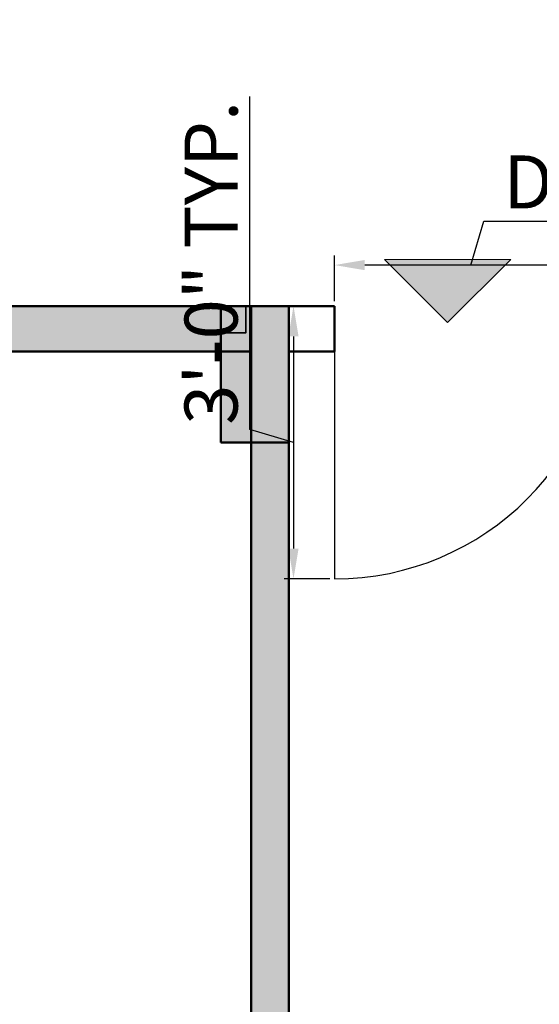
# Model space of a CAD drawing. Units: inches. Extents: x -7 to 1228, y -146 to 1091.
# Tile 14 of 88: x 200 to 269, y 401 to 531. Entities that reach past the tile are written whole.
import ezdxf

# ---------------------------------------------------------------- set-up
doc = ezdxf.new("R2010")
doc.units = ezdxf.units.IN
for name, color, linetype, lineweight in [('A-ANNO-DIMS', 2, 'Continuous', 18), ('A-ANNO-SYMB', 30, 'Continuous', 18), ('A-COLS', 6, 'Continuous', 35), ('A-DOOR', 4, 'Continuous', 25), ('A-WALL', 7, 'Continuous', 50), ('A-WALL-PATT', 251, 'Continuous', 13)]:
    doc.layers.add(name, color=color, linetype=linetype, lineweight=lineweight)
doc.styles.get("Standard").update_dxf_attribs({"font": 'arial.ttf'})
doc.dimstyles.new('ISO-25', dxfattribs={"dimtxt": 7, "dimasz": 4, "dimexe": 1.25, "dimexo": 0.625, "dimtad": 1, "dimdec": 1, "dimlunit": 3, "dimtxsty": 'Standard', "dimcen": 2.5, "dimadec": 0, "dimazin": 0, "dimtfac": 1, "dimtdec": 1, "dimtmove": 1, "dimatfit": 3, "dimfxl": 1, "dimarcsym": 0})

# ---------------------------------------------------------------- blocks, each defined once
blk = doc.blocks.new('DOOR-900')
blk.add_line((36, 0), (36, 36))
blk.add_arc((36, 0), 36, 90, 180)
blk = doc.blocks.new('*D44')
at = {"layer": 'A-ANNO-DIMS', "color": 0, "lineweight": -2, "transparency": 16777216}
for p, q in [((260, 498.4), (261.74, 504.21)), ((261.74, 504.21), (352.58, 504.21)), ((242, 493.62), (242, 499.65)), ((278, 493.62), (278, 499.65)), ((274, 498.4), (246, 498.4))]:
    blk.add_line(p, q, dxfattribs=at)
at = {"layer": 'A-ANNO-DIMS', "color": 0, "transparency": 16777216}
for points in [[(246, 499.07), (246, 497.73), (242, 498.4)], [(274, 499.07), (274, 497.73), (278, 498.4)]]:
    blk.add_solid(points, dxfattribs=at)
at = {"layer": 'Defpoints', "color": 0, "transparency": 16777216}
for p in [(242, 498.4), (242, 493), (278, 493)]:
    blk.add_point(p, dxfattribs=at)
at = {"layer": 'A-ANNO-DIMS', "color": 0, "transparency": 16777216, "insert": (307.16, 508.46), "char_height": 7, "attachment_point": 5}
blk.add_mtext('DOOR D1 3\'-0" TYP.', dxfattribs=at)
blk = doc.blocks.new('*D45')
at = {"layer": 'A-ANNO-DIMS', "color": 0, "lineweight": -2, "transparency": 16777216}
for p, q in [((230.84, 476.73), (230.84, 520.64)), ((241.38, 493), (235.35, 493)), ((236.6, 489), (236.6, 461)), ((236.6, 475), (230.84, 476.73)), ((241.38, 457), (235.35, 457))]:
    blk.add_line(p, q, dxfattribs=at)
at = {"layer": 'A-ANNO-DIMS', "color": 0, "transparency": 16777216}
for points in [[(235.93, 489), (237.27, 489), (236.6, 493)], [(235.93, 461), (237.27, 461), (236.6, 457)]]:
    blk.add_solid(points, dxfattribs=at)
at = {"layer": 'Defpoints', "color": 0, "transparency": 16777216}
for p in [(242, 493), (236.6, 457), (242, 457)]:
    blk.add_point(p, dxfattribs=at)
at = {"layer": 'A-ANNO-DIMS', "color": 0, "transparency": 16777216, "insert": (226.63, 498.69), "char_height": 7, "attachment_point": 5, "rotation": 90}
blk.add_mtext('3\'-0" TYP.', dxfattribs=at)

msp = doc.modelspace()

# ---------------------------------------------------------------- hatches: boundary and pattern name
at = {"layer": 'A-ANNO-SYMB'}
h = msp.add_hatch(color=256, dxfattribs=at)
h.dxf.hatch_style = 1
h.paths.add_polyline_path([(248.61, 499.14), (256.95, 490.81), (265.29, 499.14)])
at = {"layer": 'A-COLS'}
h = msp.add_hatch(color=256, dxfattribs=at)
h.dxf.hatch_style = 1
h.paths.add_polyline_path([(227, 475), (236, 475), (236, 493), (230.29, 493), (230.29, 489.45), (227, 489.45)])
h = msp.add_hatch(color=256, dxfattribs=at)
h.dxf.hatch_style = 1
h.paths.add_polyline_path([(230.29, 489.45), (230.29, 493), (227, 493), (227, 489.45)])
at = {"layer": 'A-WALL-PATT'}
h = msp.add_hatch(color=256, dxfattribs=at)
h.dxf.hatch_style = 1
h.paths.add_polyline_path([(69, 568), (60, 568), (60, 493), (63.29, 493), (69, 493)])
h.paths.add_polyline_path([(69, 662.41), (60, 662.41), (60, 586), (69, 586)], flags=17)
h.paths.add_polyline_path([(69, 723), (184, 723), (184, 734), (179, 734), (179, 728), (69, 728), (69, 741.62), (60, 741.62), (60, 698.41), (69, 698.41)], flags=17)
h.paths.add_polyline_path([(69, 782), (231, 782), (231, 728), (231, 723), (231, 586), (236, 586), (236, 787), (69, 787), (69, 800.13), (60, 800.13), (60, 765.62), (69, 765.62)])
h.paths.add_polyline_path([(184, 842), (189, 842), (189, 848), (173, 848), (173, 842), (179, 842), (179, 787), (184, 787)])
h.paths.add_polyline_path([(118.22, 69), (69, 69), (69, 60), (118.22, 60)])
h.paths.add_polyline_path([(227, 69), (154.22, 69), (154.22, 60), (227, 60)])
h.paths.add_polyline_path([(236, 60), (232.71, 60), (227, 60), (227, 36), (236, 36)])
h.paths.add_polyline_path([(389, 60), (380, 60), (380, 36), (389, 36)])
h.paths.add_polyline_path([(384, 181), (380, 181), (380, 115), (380, 78), (384, 78)])
h.paths.add_polyline_path([(380, 115), (334.55, 115), (334.55, 109), (380, 109)])
h.paths.add_polyline_path([(274.55, 115), (236, 115), (236, 201), (232.71, 201), (231, 201), (231, 78), (236, 78), (236, 109), (274.55, 109)])
h.paths.add_polyline_path([(69, 123), (60, 123), (60, 78), (69, 78)])
h.paths.add_polyline_path([(69, 201), (60, 201), (60, 159), (69, 159)])
h.paths.add_polyline_path([(143, 219), (69, 219), (69, 213), (143, 213)], flags=17)
h.paths.add_polyline_path([(189, 219), (184, 219), (184, 274), (231, 274), (231, 219), (236, 219), (236, 279), (184, 279), (184, 297), (179, 297), (179, 279), (69, 279), (69, 290.91), (60, 290.91), (60, 262.18), (69, 262.18), (69, 274), (179, 274), (179, 219), (173, 219), (173, 213), (189, 213)])
h.paths.add_polyline_path([(69, 238.18), (60, 238.18), (60, 219), (69, 219)], flags=17)
h.paths.add_polyline_path([(69, 333), (60, 333), (60, 314.91), (69, 314.91), (69, 316.96)])
h.paths.add_polyline_path([(190, 338), (184, 338), (69, 338), (69, 333), (179, 333), (179, 327), (184, 327), (184, 333.02), (190, 333.05)])
h.paths.add_polyline_path([(69, 386.81), (60, 386.81), (60, 351), (69, 351)])
h.paths.add_polyline_path([(69, 475), (60, 475), (60, 422.81), (69, 422.81)])
h.paths.add_polyline_path([(236, 475), (231, 475), (231, 351.24), (236, 351.24)])
h.paths.add_polyline_path([(384, 475), (380, 475), (380, 362), (384, 362)])
h.paths.add_polyline_path([(547, 307), (439, 307), (439, 356), (445, 356), (445, 362), (433, 362), (433, 307), (380, 307), (380, 244), (380, 241), (384, 241), (384, 301), (433, 301), (433, 277), (439, 277), (439, 301), (547, 301)])
h.paths.add_polyline_path([(547, 241), (439, 241), (439, 247), (433, 247), (433, 235), (547, 235)])
h.paths.add_polyline_path([(450, 69), (440.29, 69), (424.89, 69), (389, 69), (389, 60), (450, 60)])
h.paths.add_polyline_path([(547, 69), (486, 69), (486, 60), (547, 60)])
h.paths.add_polyline_path([(556, 148.27), (547, 148.27), (547, 78), (556, 78)])
h.paths.add_polyline_path([(556, 223), (547, 223), (547, 195), (547, 184.27), (556, 184.27)])
h.paths.add_polyline_path([(556, 311.19), (547, 311.19), (547, 273.08), (556, 273.08)])
h.paths.add_polyline_path([(556, 344), (552.71, 344), (547, 344), (547, 335.19), (556, 335.19)])
h.paths.add_polyline_path([(556, 249.08), (547, 249.08), (547, 241), (556, 241)])
h.paths.add_polyline_path([(547, 362), (475, 362), (475, 356), (547, 356)], flags=0)
h.paths.add_polyline_path([(556, 399.62), (547, 399.62), (547, 362), (556, 362)])
h.paths.add_polyline_path([(556, 475), (547, 475), (547, 435.62), (556, 435.62)])
h.paths.add_polyline_path([(547, 493), (389, 493), (389, 487), (547, 487)])
h.paths.add_polyline_path([(380, 493), (278, 493), (278, 487), (380, 487)])
h.paths.add_polyline_path([(227, 493), (69, 493), (69, 487), (227, 487)])
h.paths.add_polyline_path([(643, 122.44), (634, 122.44), (634, 78), (643, 78)])
h.paths.add_polyline_path([(702.5, 69), (692.79, 69), (677.39, 69), (643, 69), (643, 60), (702.5, 60)])
h.paths.add_polyline_path([(798, 69), (738.5, 69), (738.5, 60), (798, 60)])
h.paths.add_polyline_path([(807, 60), (803.71, 60), (798, 60), (798, 36), (807, 36)])
h.paths.add_polyline_path([(807, 109), (846.75, 109), (846.75, 115), (807, 115), (807, 159), (802, 159), (802, 78), (807, 78)])
h.paths.add_polyline_path([(807, 201), (802, 201), (802, 195), (807, 195)])
h.paths.add_polyline_path([(643, 201), (634, 201), (634, 158.44), (643, 158.44)])
h.paths.add_polyline_path([(756, 225), (751, 225), (751, 219), (643, 219), (643, 213), (756, 213)])
h.paths.add_polyline_path([(643, 240.85), (634, 240.85), (634, 219), (643, 219)])
h.paths.add_polyline_path([(643, 274), (643, 288.63), (634, 288.63), (634, 264.85), (643, 264.85)])
h.paths.add_polyline_path([(802, 279), (756, 279), (756, 297), (751, 297), (751, 279), (643, 279), (643, 274), (751, 274), (751, 255), (756, 255), (756, 274), (802, 274)])
h.paths.add_polyline_path([(807, 333), (803.71, 333), (802, 333), (802, 279), (802, 274), (802, 219), (807, 219)])
h.paths.add_polyline_path([(956, 182), (951, 182), (951, 115), (906.75, 115), (906.75, 109), (951, 109), (951, 78), (956, 78)])
h.paths.add_polyline_path([(960, 60), (951, 60), (951, 36), (960, 36)])
h.paths.add_polyline_path([(1021, 69), (1005.78, 69), (960, 69), (960, 60), (1021, 60)])
h.paths.add_polyline_path([(956, 224), (951, 224), (951, 218), (956, 218)])
h.paths.add_polyline_path([(956, 302), (1004, 302), (1004, 278), (1010, 278), (1010, 302), (1118, 302), (1118, 290.81), (1127, 290.81), (1127, 326.97), (1118, 326.97), (1118, 320.97), (1118, 307), (1010, 307), (1010, 356), (1016, 356), (1016, 362), (1004, 362), (1004, 307), (951, 307), (951, 244), (951, 242), (954.29, 242), (956, 242)])
h.paths.add_polyline_path([(643, 333), (634, 333), (634, 312.63), (643, 312.63), (643, 316.96)])
h.paths.add_polyline_path([(756, 338), (643, 338), (643, 333), (751, 333), (751, 327), (756, 327)])
h.paths.add_polyline_path([(643, 388), (634, 388), (634, 351), (643, 351)])
h.paths.add_polyline_path([(807, 357), (802, 357), (802, 351), (807, 351)])
h.paths.add_polyline_path([(807, 475), (802, 475), (802, 393), (807, 393)])
h.paths.add_polyline_path([(643, 475), (634, 475), (634, 424), (643, 424)])
h.paths.add_polyline_path([(798, 493), (643, 493), (643, 487), (798, 487)])
h.paths.add_polyline_path([(634, 493), (556, 493), (556, 487), (634, 487)])
h.paths.add_polyline_path([(813, 493), (807, 493), (807, 487), (813, 487)])
h.paths.add_polyline_path([(951, 493), (849, 493), (849, 487), (951, 487)])
h.paths.add_polyline_path([(956, 484), (951, 484), (951, 374), (956, 374)])
h.paths.add_polyline_path([(1109, 493), (969, 493), (969, 487), (1109, 487)])
h.paths.add_polyline_path([(1127, 484), (1118, 484), (1118, 450.64), (1127, 450.64)])
h.paths.add_polyline_path([(1127, 414.64), (1118, 414.64), (1118, 365), (1127, 365)])
h.paths.add_polyline_path([(1109, 362), (1046, 362), (1046, 356), (1109, 356)], flags=17)
h.paths.add_polyline_path([(1127, 356), (1123.45, 356), (1118, 356), (1118, 350.97), (1127, 350.97)], flags=0)
h.paths.add_polyline_path([(1127, 266.81), (1118, 266.81), (1118, 262.36), (1118, 242), (1127, 242)], flags=17)
h.paths.add_polyline_path([(1118, 242), (1010, 242), (1010, 248), (1004, 248), (1004, 237), (1118, 237)])
h.paths.add_polyline_path([(1127, 224), (1118, 224), (1118, 170), (1127, 170)])
h.paths.add_polyline_path([(1127, 134), (1118, 134), (1118, 78), (1127, 78)])
h.paths.add_polyline_path([(1118, 69), (1057, 69), (1057, 60), (1118, 60)])
h.paths.add_polyline_path([(227, 571.55), (227, 574), (69, 574), (69, 568), (227, 568)])
h.paths.add_polyline_path([(380, 571.55), (380, 574), (278, 574), (278, 568), (380, 568)])
h.paths.add_polyline_path([(242, 574), (236, 574), (236, 568), (242, 568)])
h.paths.add_polyline_path([(547, 571.55), (547, 574), (389, 574), (389, 568), (547, 568)])
h.paths.add_polyline_path([(384, 733), (380, 733), (380, 586), (384, 586)])
h.paths.add_polyline_path([(556, 646), (634, 646), (634, 655), (547, 655), (547, 586), (556, 586)])
h.paths.add_polyline_path([(634, 574), (556, 574), (556, 568), (634, 568)])
h.paths.add_polyline_path([(643, 655), (634, 655), (634, 586), (643, 586)])
h.paths.add_polyline_path([(798, 574), (643, 574), (643, 568), (798, 568)])
h.paths.add_polyline_path([(643, 663.85), (634, 663.85), (634, 655), (643, 655)])
h.paths.add_polyline_path([(556, 676.97), (547, 676.97), (547, 655), (556, 655)])
h.paths.add_polyline_path([(556, 733), (547, 733), (547, 712.97), (556, 712.97)])
h.paths.add_polyline_path([(643, 710), (634, 710), (634, 699.85), (643, 699.85)])
h.paths.add_polyline_path([(807, 668), (802, 668), (802, 586), (807, 586)])
h.paths.add_polyline_path([(951, 574), (849, 574), (849, 568), (951, 568)])
h.paths.add_polyline_path([(956, 691), (951, 691), (951, 577), (956, 577)])
h.paths.add_polyline_path([(1109, 574), (969, 574), (969, 568), (1109, 568)])
h.paths.add_polyline_path([(1127, 643.4), (1118, 643.4), (1118, 577), (1127, 577)])
h.paths.add_polyline_path([(1127, 568), (1123.45, 568), (1118, 568), (1118, 493), (1127, 493)])
h.paths.add_polyline_path([(1127, 733), (1118, 733), (1118, 679.4), (1127, 679.4)])
h.paths.add_polyline_path([(1127, 777.35), (1118, 777.35), (1118, 770.04), (1118, 751), (1127, 751)], flags=17)
h.paths.add_polyline_path([(1118, 751), (1010, 751), (1010, 757), (1004, 757), (1004, 745), (1118, 745)])
h.paths.add_polyline_path([(956, 811), (1004, 811), (1004, 787), (1010, 787), (1010, 811), (1017.87, 811), (1017.87, 811.63, -0.414214), (1018.25, 812), (1031.98, 812, -0.414214), (1032.35, 811.63), (1032.35, 811), (1118, 811), (1118, 801.35), (1127, 801.35), (1127, 834.69), (1118, 834.69), (1118, 830.24), (1118, 817), (1010, 817), (1010, 866), (1016, 866), (1016, 872), (1004, 872), (1004, 817), (956, 817), (956, 866), (951, 866), (951, 751), (954.29, 751), (956, 751)])
h.paths.add_polyline_path([(1118, 872), (1046, 872), (1046, 866), (1118, 866)], flags=17)
h.paths.add_polyline_path([(1127, 924.71), (1118, 924.71), (1118, 884), (1127, 884)])
h.paths.add_polyline_path([(1127, 866), (1123.71, 866), (1118, 866), (1118, 858.69), (1127, 858.69)], flags=17)
h.paths.add_polyline_path([(956, 983), (951, 983), (951, 952), (807, 952), (807, 983), (802, 983), (802, 902), (807, 902), (807, 946), (951, 946), (951, 884), (956, 884)])
h.paths.add_polyline_path([(807, 842), (802, 842), (802, 787), (756, 787), (756, 806), (751, 806), (751, 787), (643, 787), (643, 782), (751, 782), (751, 764), (756, 764), (756, 782), (802, 782), (802, 728), (807, 728)])
h.paths.add_polyline_path([(756, 848), (643, 848), (643, 842), (751, 842), (751, 836), (756, 836)])
h.paths.add_polyline_path([(756, 734), (751, 734), (751, 728), (643, 728), (643, 723), (756, 723)])
h.paths.add_polyline_path([(643, 749.79), (634, 749.79), (634, 728), (637.29, 728), (643, 728)])
h.paths.add_polyline_path([(643, 805.41), (634, 805.41), (634, 773.79), (643, 773.79)])
h.paths.add_polyline_path([(643, 896.66), (634, 896.66), (634, 860), (637.29, 860), (643, 860)])
h.paths.add_polyline_path([(643, 842), (634, 842), (634, 829.41), (643, 829.41)])
h.paths.add_polyline_path([(643, 983), (634, 983), (634, 932.66), (643, 932.66)])
h.paths.add_polyline_path([(1127, 983), (1118, 983), (1118, 960.71), (1127, 960.71)])
h.paths.add_polyline_path([(1118, 1001), (1077.53, 1001), (1077.53, 992), (1118, 992)])
h.paths.add_polyline_path([(1041.53, 1001), (960, 1001), (960, 992), (1041.53, 992)])
h.paths.add_polyline_path([(960, 1025), (951, 1025), (951, 1001), (954.29, 1001), (960, 1001)])
h.paths.add_polyline_path([(807, 1025), (798, 1025), (798, 1001), (807, 1001)])
h.paths.add_polyline_path([(798, 1001), (738.5, 1001), (738.5, 992), (798, 992)])
h.paths.add_polyline_path([(702.5, 1001), (643, 1001), (643, 992), (702.5, 992)])
h.paths.add_polyline_path([(547, 1001), (499.11, 1001), (499.11, 992), (547, 992)])
h.paths.add_polyline_path([(463.11, 1001), (389, 1001), (389, 992), (463.11, 992)])
h.paths.add_polyline_path([(389, 1025), (380, 1025), (380, 1022), (380, 1001), (383.29, 1001), (389, 1001)])
h.paths.add_polyline_path([(236, 1025), (227, 1025), (227, 1001), (236, 1001)])
h.paths.add_polyline_path([(236, 983), (231, 983), (231, 860), (236, 860)])
h.paths.add_polyline_path([(274.55, 952), (236, 952), (236, 946), (274.55, 946)])
h.paths.add_polyline_path([(380, 952), (334.55, 952), (334.55, 946), (380, 946)])
h.paths.add_polyline_path([(384, 983), (380, 983), (380, 884), (383.29, 884), (384, 884)])
h.paths.add_polyline_path([(227, 1001), (155.01, 1001), (155.01, 992), (162.87, 992), (227, 992)])
h.paths.add_polyline_path([(119.01, 1001), (69, 1001), (69, 992), (119.01, 992)])
h.paths.add_polyline_path([(69, 983), (60, 983), (60, 922.99), (69, 922.99)])
h.paths.add_polyline_path([(69, 886.99), (60, 886.99), (60, 860), (63.29, 860), (69, 860)])
h.paths.add_polyline_path([(143, 848), (69, 848), (69, 842), (143, 842)])

# ---------------------------------------------------------------- linework, layer by layer
at = {"layer": 'A-ANNO-SYMB'}
for p, q in [((256.95, 490.81), (248.61, 499.14)), ((248.61, 499.14), (265.29, 499.14)), ((256.95, 490.81), (265.29, 499.14))]:
    msp.add_line(p, q, dxfattribs=at)
at = {"layer": 'A-COLS'}
msp.add_lwpolyline([(227, 493), (230.29, 493), (230.29, 489.45), (227, 489.45)], close=True, dxfattribs=at)
at = {"layer": 'A-WALL'}
for p, q in [((231, 493), (60, 493)), ((227, 493), (236, 493)), ((227, 475), (227, 493)), ((231, 493), (231, 333.22)), ((236, 493), (236, 333.24)), ((242, 493), (236, 493)), ((236, 493), (236, 475)), ((242, 487), (242, 493)), ((231, 487), (69, 487)), ((231, 338), (231, 487)), ((242, 487), (236, 487)), ((236, 333.24), (236, 487)), ((236, 475), (227, 475))]:
    msp.add_line(p, q, dxfattribs=at)

# ---------------------------------------------------------------- block references
at = {"layer": 'A-DOOR', "rotation": 180}
msp.add_blockref('DOOR-900', (278, 493), dxfattribs=at)

# ---------------------------------------------------------------- dimensions: what is measured, and where the dimension line sits
at = {"layer": 'A-ANNO-DIMS'}
for base, p1, p2, angle, text, picture, middle in [((242, 498.4), (278, 493), (242, 493), 180, 'DOOR D1 <> TYP.', '*D44', (262.37, 508.46)), ((236.6, 457), (242, 493), (242, 457), 270, '<> TYP.', '*D45', (226.63, 477.35))]:
    dim = msp.add_linear_dim(base=base, p1=p1, p2=p2, angle=angle, text=text, dimstyle='ISO-25', override={"dimdec": 1, "dimlfac": 1, "dimrnd": 0, "dimzin": 1, "dimdsep": 46, "dimlunit": 4, "dimfrac": 2}, dxfattribs=at)
    dim.commit()
    dim.dimension.update_dxf_attribs({"geometry": picture, "text_midpoint": middle})

doc.saveas('drawing.dxf')
